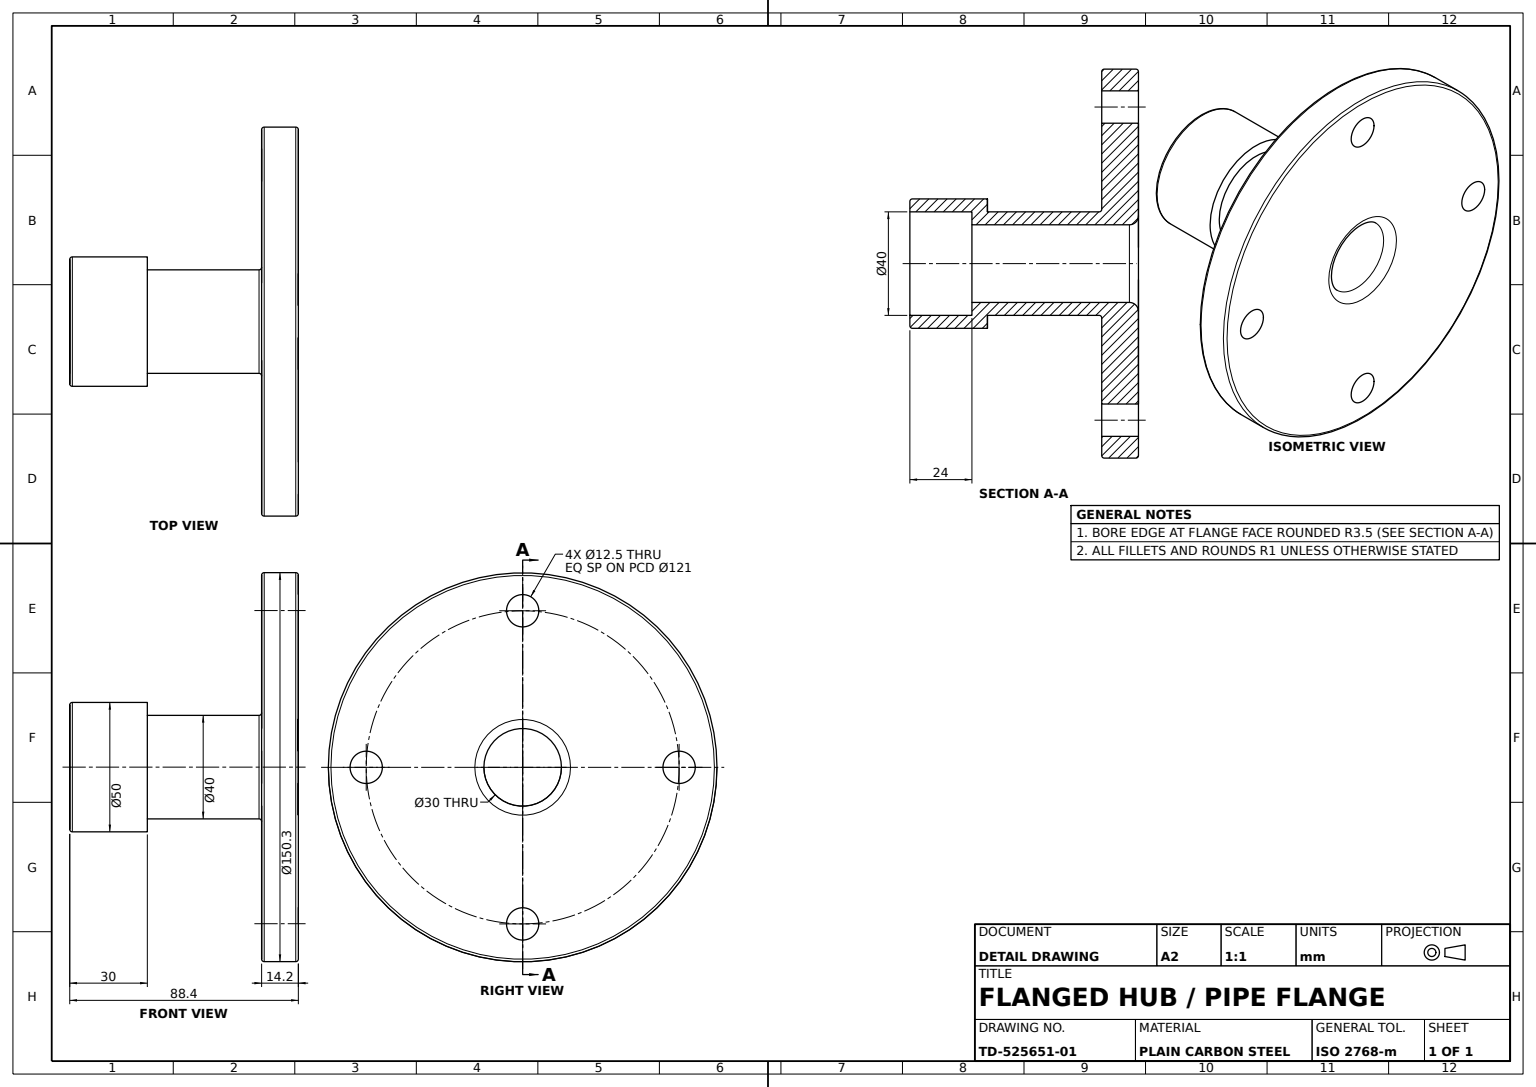
from build123d import *

# Parameters (mm, degrees)
BOLT_HOLES_SKETCH_R        = 6.25
FLANGE_BOLT_HOLES_4X_DEPTH = 52
FILLET_R3_5_R              = 3.5
FILLET_R1_R                = 1


with BuildPart() as part:
    # Connector Profile Sketch → Connector Body Revolve (revolve)
    with BuildSketch(Plane.XY, mode=Mode.PRIVATE) as connector_body_revolve_sk:
        Polygon((0, 25), (30, 25), (30, 20), (74.2, 20), (74.2, 75.14842088), (88.4, 75.14842088), (88.4, 15), (24, 15), (24, 20), (0, 20), align=None)
    revolve(connector_body_revolve_sk.sketch.rotate(Axis((-1000, 0, 0), (1, 0, 0)), 90), axis=Axis((-1000, 0, 0), (1, 0, 0)))

    # Bolt Holes Sketch → Flange Bolt Holes 4x (cut)
    with BuildSketch(Plane.ZY.offset(-74.2)):
        with Locations((0, 60.5)):
            Circle(BOLT_HOLES_SKETCH_R)
        with Locations((0, -60.5)):
            Circle(BOLT_HOLES_SKETCH_R)
        with Locations((-60.5, 0)):
            Circle(BOLT_HOLES_SKETCH_R)
        with Locations((60.5, 0)):
            Circle(BOLT_HOLES_SKETCH_R)
    extrude(amount=-FLANGE_BOLT_HOLES_4X_DEPTH, mode=Mode.SUBTRACT)

    # Fillet R3.5
    fillet_r3_5_edges = [part.edges().sort_by_distance(p)[0] for p in [
        (88.4, 0, -15),
    ]]
    fillet(fillet_r3_5_edges, radius=FILLET_R3_5_R)

    # Fillet R1
    fillet_r1_edges = [part.edges().sort_by_distance(p)[0] for p in [
        (74.2, 0, -75.14842088),
        (74.2, 0, -20),
        (0, 0, -25),
        (88.4, 0, -75.14842088),
    ]]
    fillet(fillet_r1_edges, radius=FILLET_R1_R)


solid = part.part
